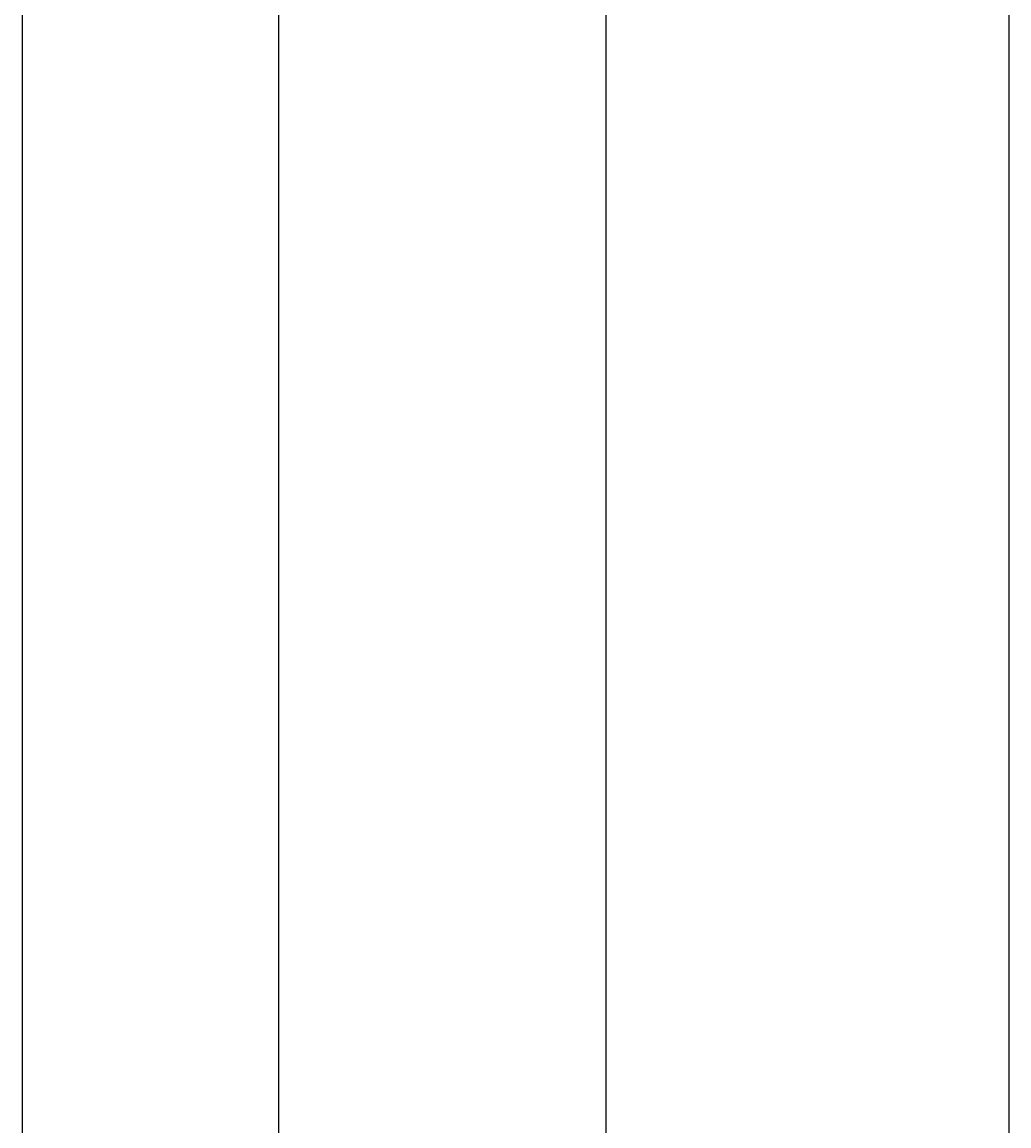
# Model space of a CAD drawing. Units: inches. Extents: x 2812 to 3051, y 1398 to 1659.
# Tile 43 of 65: x 3011 to 3038, y 1498 to 1528. Entities that reach past the tile are written whole.
import ezdxf

# ---------------------------------------------------------------- set-up
doc = ezdxf.new("R2010")
doc.units = ezdxf.units.IN
doc.layers.add('A-ANNO-DIMS', color=2, linetype='Continuous', lineweight=18)
doc.styles.get("Standard").update_dxf_attribs({"font": 'arial.ttf'})
doc.dimstyles.get("Standard").update_dxf_attribs({"dimtxt": 0.18, "dimasz": 0.18, "dimexe": 0.18, "dimexo": 0.0625, "dimgap": 0.09, "dimtad": 0, "dimtih": 1, "dimtoh": 1, "dimdec": 4, "dimzin": 0, "dimdsep": 46, "dimtxsty": 'Standard', "dimcen": 0.09, "dimadec": 0, "dimazin": 0, "dimtfac": 1, "dimtdec": 4, "dimtofl": 0, "dimtmove": 0, "dimatfit": 3, "dimfxl": 1, "dimtolj": 1, "dimtzin": 0, "dimarcsym": 0})

# ---------------------------------------------------------------- blocks, each defined once
blk = doc.blocks.new('*D33')
at = {"layer": 'A-ANNO-DIMS', "color": 0, "lineweight": -2, "transparency": 16777216}
for p, q in [((3011.337, 1597.982), (3011.337, 1397.505)), ((3018.385, 1559.757), (3018.385, 1397.505)), ((3011.517, 1397.685), (3014.468, 1397.685)), ((3018.205, 1397.685), (3015.254, 1397.685))]:
    blk.add_line(p, q, dxfattribs=at)
at = {"layer": 'A-ANNO-DIMS', "color": 0, "transparency": 16777216}
for points in [[(3011.517, 1397.715), (3011.517, 1397.655), (3011.337, 1397.685)], [(3018.205, 1397.715), (3018.205, 1397.655), (3018.385, 1397.685)]]:
    blk.add_solid(points, dxfattribs=at)
at = {"layer": 'Defpoints', "color": 0, "transparency": 16777216}
for p in [(3011.337, 1598.044), (3018.385, 1559.82), (3018.385, 1397.685)]:
    blk.add_point(p, dxfattribs=at)
at = {"layer": 'A-ANNO-DIMS', "color": 0, "transparency": 16777216, "insert": (3014.861, 1397.685), "char_height": 0.18, "attachment_point": 5}
blk.add_mtext('\\A1;7.048', dxfattribs=at)
blk = doc.blocks.new('*D34')
at = {"layer": 'A-ANNO-DIMS', "color": 0, "lineweight": -2, "transparency": 16777216}
for p, q in [((3038.462, 1593.482), (3038.462, 1397.505)), ((3027.385, 1550.757), (3027.385, 1397.505)), ((3027.565, 1397.685), (3032.468, 1397.685)), ((3038.282, 1397.685), (3033.379, 1397.685))]:
    blk.add_line(p, q, dxfattribs=at)
at = {"layer": 'A-ANNO-DIMS', "color": 0, "transparency": 16777216}
for points in [[(3027.565, 1397.715), (3027.565, 1397.655), (3027.385, 1397.685)], [(3038.282, 1397.715), (3038.282, 1397.655), (3038.462, 1397.685)]]:
    blk.add_solid(points, dxfattribs=at)
at = {"layer": 'Defpoints', "color": 0, "transparency": 16777216}
for p in [(3038.462, 1593.544), (3027.385, 1550.82), (3038.462, 1397.685)]:
    blk.add_point(p, dxfattribs=at)
at = {"layer": 'A-ANNO-DIMS', "color": 0, "transparency": 16777216, "insert": (3032.923, 1397.685), "char_height": 0.18, "attachment_point": 5}
blk.add_mtext('\\A1;11.077', dxfattribs=at)

msp = doc.modelspace()

# ---------------------------------------------------------------- dimensions: what is measured, and where the dimension line sits
at = {"layer": 'A-ANNO-DIMS'}
for base, p1, p2, picture, middle in [((3018.3849, 1397.6854), (3011.3373, 1598.0441), (3018.3849, 1559.82), '*D33', (3014.8611, 1397.6854)), ((3038.4621, 1397.6854), (3027.3849, 1550.82), (3038.4621, 1593.5441), '*D34', (3032.9235, 1397.6854))]:
    dim = msp.add_linear_dim(base=base, p1=p1, p2=p2, dimstyle='Standard', override={"dimdec": 3, "dimlfac": 1, "dimrnd": 0, "dimzin": 0, "dimdsep": 46, "dimlunit": 2}, dxfattribs=at)
    dim.commit()
    dim.dimension.update_dxf_attribs({"geometry": picture, "text_midpoint": middle})

doc.saveas('drawing.dxf')
